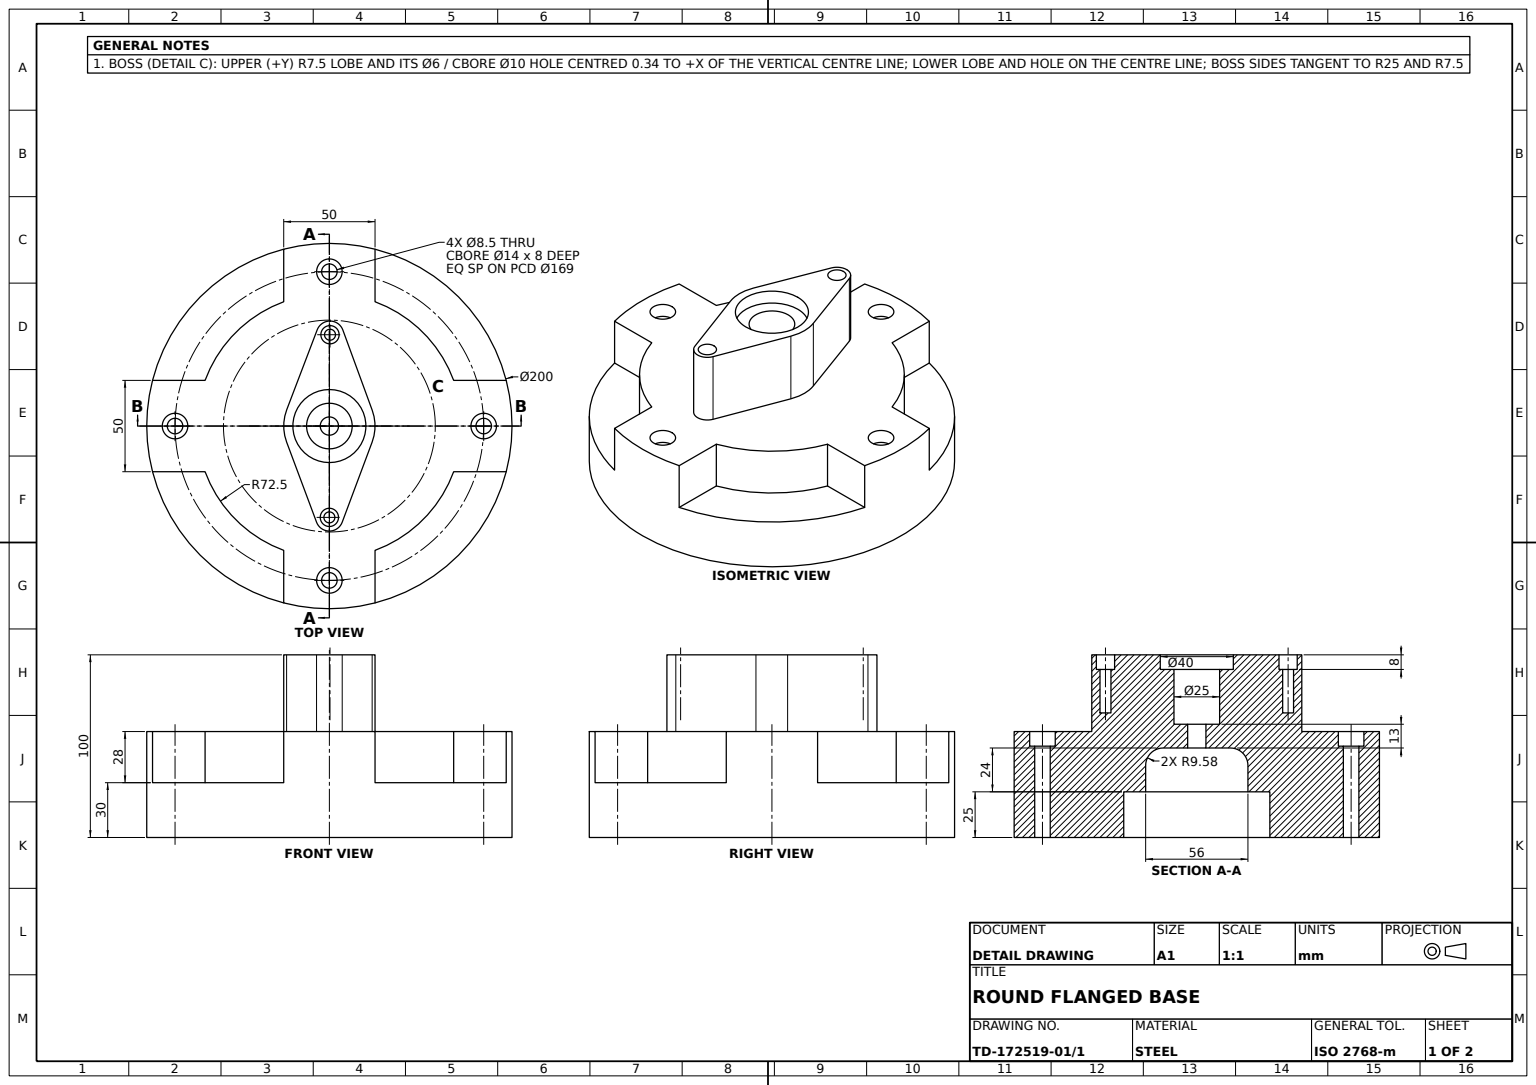
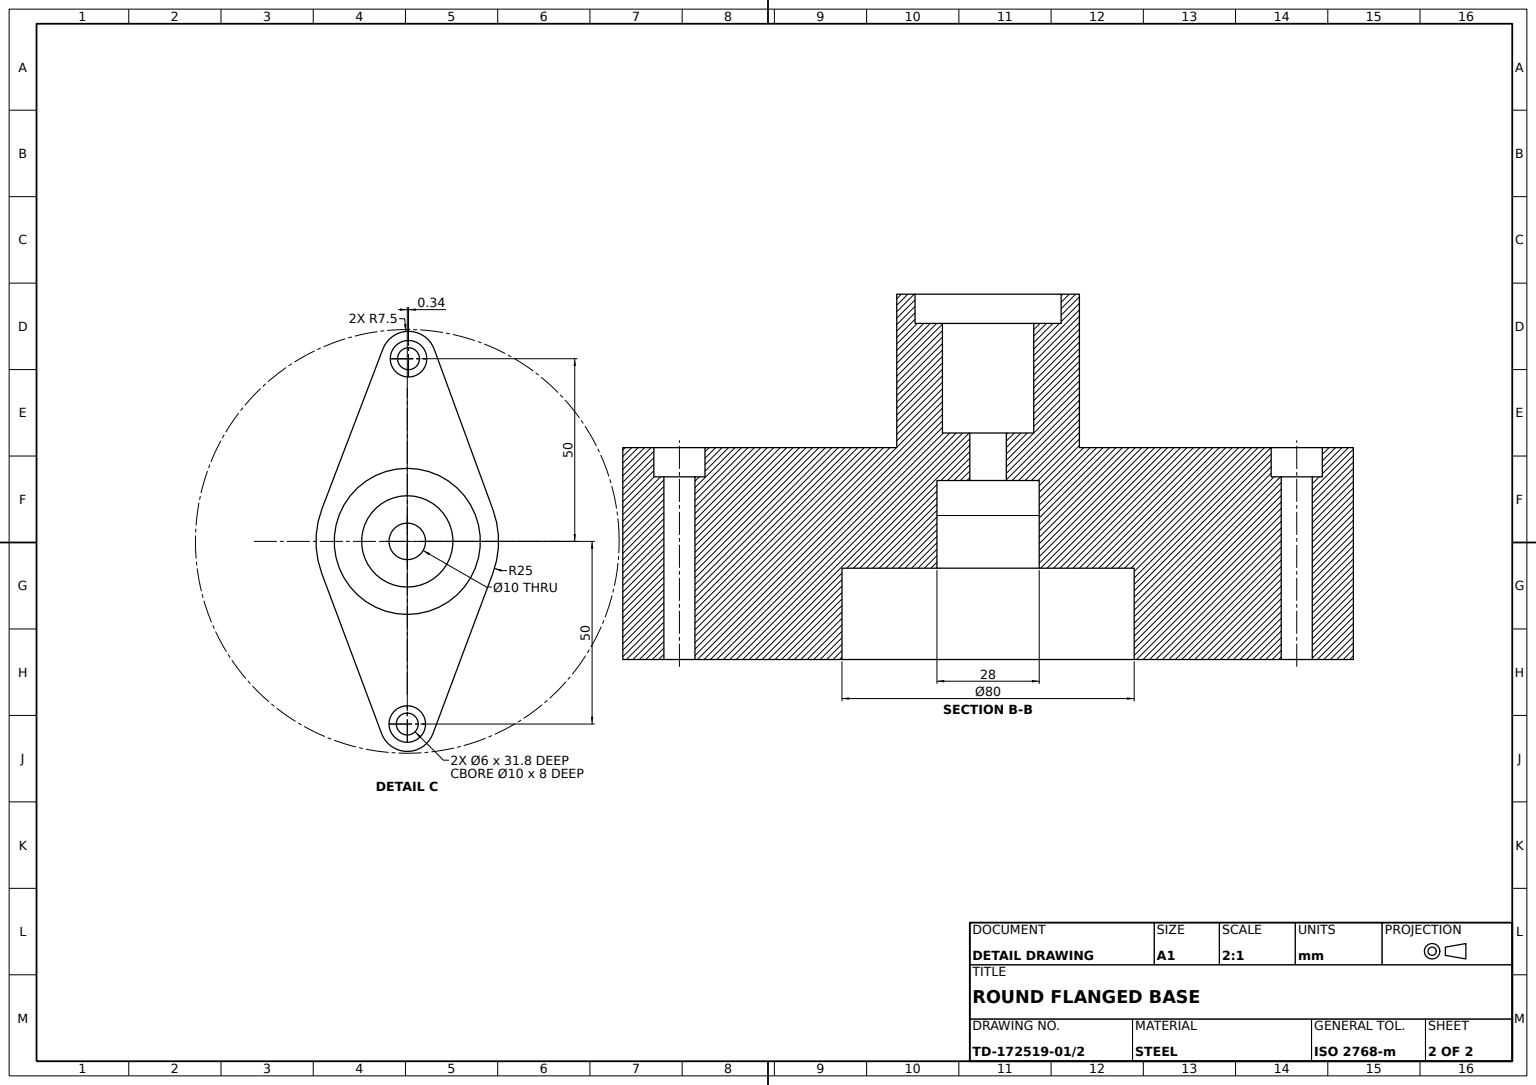
from build123d import *
from build123d.topology import SkipClean

# Parameters (mm, degrees)
BASE_FLANGE_SKETCH_R               = 100
BASE_FLANGE_200_DEPTH              = 30
MOUNTING_PAD_DEPTH                 = 28
MOUNTING_COUNTERBORES_SKETCH_R     = 7
MOUNTING_COUNTERBORES_4X_14_DEPTH  = 8
MOUNTING_HOLES_SKETCH_R            = 4.25
MOUNTING_HOLES_4X_8_5_DEPTH        = 50
SUPPORT_BOSS_DEPTH                 = 42
BEARING_COUNTERBORE_SKETCH_R       = 20
BEARING_COUNTERBORE_40_DEPTH       = 8
BEARING_BORE_SKETCH_R              = 12.5
BEARING_BORE_25_DEPTH              = 30
THROUGH_BORE_SKETCH_R              = 5
THROUGH_BORE_10_DEPTH              = 13
UNDERSIDE_RECESS_SKETCH_R          = 40
UNDERSIDE_RECESS_80_DEPTH          = 25
SIDE_SLOT_DEPTH                    = 14
BOSS_HOLE_COUNTERBORES_SKETCH_R    = 5
BOSS_HOLE_COUNTERBORES_2X_10_DEPTH = 8
BOSS_PIN_HOLES_SKETCH_R            = 3
BOSS_PIN_HOLES_2X_6_DEPTH          = 23.8


with BuildPart() as part:
    # Base Flange Sketch → Base Flange Ø200 (new body)
    with BuildSketch(Plane(origin=(0, 0, 0), x_dir=(1, 0, 0), z_dir=(0, 1, 0))):
        with Locations(Location((0, 0, 0), (0, 0, 270))):
            Circle(BASE_FLANGE_SKETCH_R)
    extrude(amount=BASE_FLANGE_200_DEPTH)

    # Mounting Pad Sketch → Mounting Pad (add)
    with SkipClean():  # the faces are left unmerged after this step: merging them gives an invalid solid
        with BuildSketch(Plane(origin=(0, 30, 0), x_dir=(1, 0, 0), z_dir=(0, 1, 0))):
            with BuildLine():
                Line((68.053287944, 25), (96.824583655, 25))
                ThreePointArc((96.824583655, 25), (100, 0), (96.824583655, -25))
                Line((96.824583655, -25), (68.053287944, -25))
                ThreePointArc((68.053287944, -25), (51.265241636, -51.265241636), (25, -68.053287944))
                Line((25, -68.053287944), (25, -96.824583655))
                ThreePointArc((25, -96.824583655), (0, -100), (-25, -96.824583655))
                Line((-25, -96.824583655), (-25, -68.053287944))
                ThreePointArc((-25, -68.053287944), (-51.265241636, -51.265241636), (-68.053287944, -25))
                Line((-68.053287944, -25), (-96.824583655, -25))
                ThreePointArc((-96.824583655, -25), (-100, 0), (-96.824583655, 25))
                Line((-96.824583655, 25), (-68.053287944, 25))
                ThreePointArc((-68.053287944, 25), (-51.265241636, 51.265241636), (-25, 68.053287944))
                Line((-25, 68.053287944), (-25, 96.824583655))
                ThreePointArc((-25, 96.824583655), (0, 100), (25, 96.824583655))
                Line((25, 96.824583655), (25, 68.053287944))
                ThreePointArc((25, 68.053287944), (51.265241636, 51.265241636), (68.053287944, 25))
            make_face()
        extrude(amount=MOUNTING_PAD_DEPTH)

    # Mounting Counterbores Sketch → Mounting Counterbores 4xØ14 (cut)
    with SkipClean():  # the faces are left unmerged after this step: merging them gives an invalid solid
        with BuildSketch(Plane(origin=(0, 58, 0), x_dir=(1, 0, 0), z_dir=(0, 1, 0))):
            with Locations(Location((0, 84.5, 0), (0, 0, 270))):
                Circle(MOUNTING_COUNTERBORES_SKETCH_R)
            with Locations(Location((84.5, 0, 0), (0, 0, 270))):
                Circle(MOUNTING_COUNTERBORES_SKETCH_R)
            with Locations(Location((0, -84.5, 0), (0, 0, 270))):
                Circle(MOUNTING_COUNTERBORES_SKETCH_R)
            with Locations(Location((-84.5, 0, 0), (0, 0, 270))):
                Circle(MOUNTING_COUNTERBORES_SKETCH_R)
        extrude(amount=-MOUNTING_COUNTERBORES_4X_14_DEPTH, mode=Mode.SUBTRACT)

    # Mounting Holes Sketch → Mounting Holes 4xØ8.5 (cut)
    with SkipClean():  # the faces are left unmerged after this step: merging them gives an invalid solid
        with BuildSketch(Plane(origin=(0, 50, 0), x_dir=(1, 0, 0), z_dir=(0, 1, 0))):
            with Locations(Location((0, 84.5, 0), (0, 0, 270))):
                Circle(MOUNTING_HOLES_SKETCH_R)
            with Locations(Location((84.5, 0, 0), (0, 0, 270))):
                Circle(MOUNTING_HOLES_SKETCH_R)
            with Locations(Location((0, -84.5, 0), (0, 0, 270))):
                Circle(MOUNTING_HOLES_SKETCH_R)
            with Locations(Location((-84.5, 0, 0), (0, 0, 270))):
                Circle(MOUNTING_HOLES_SKETCH_R)
        extrude(amount=-MOUNTING_HOLES_4X_8_5_DEPTH, mode=Mode.SUBTRACT)

    # Support Boss Sketch → Support Boss (add)
    with SkipClean():  # the faces are left unmerged after this step: merging them gives an invalid solid
        with BuildSketch(Plane(origin=(0, 58, 0), x_dir=(1, 0, 0), z_dir=(0, 1, 0))):
            with BuildLine():
                Line((-6.670404666, 52.671203723), (-23.359173661, 8.907805895))
                ThreePointArc((-23.359173661, 8.907805895), (-24.999857744, 0.084337338), (-23.418742494, -8.75))
                Line((-23.418742494, -8.75), (-7.025622749, -52.625))
                ThreePointArc((-7.025622749, -52.625), (-1e-09, -57.5), (7.025622747, -52.625))
                Line((7.025622747, -52.625), (23.418742494, -8.75))
                ThreePointArc((23.418742494, -8.75), (24.999857744, -0.084337338), (23.477245263, 8.591795789))
                Line((23.477245263, 8.591795789), (7.380521011, 52.576400691))
                ThreePointArc((7.380521011, 52.576400691), (0.387949547, 57.498691247), (-6.670404666, 52.671203723))
            make_face()
        extrude(amount=SUPPORT_BOSS_DEPTH)

    # Bearing Counterbore Sketch → Bearing Counterbore Ø40 (cut)
    with SkipClean():  # the faces are left unmerged after this step: merging them gives an invalid solid
        with BuildSketch(Plane(origin=(0, 100, 0), x_dir=(1, 0, 0), z_dir=(0, 1, 0))):
            with Locations(Location((0, 0, 0), (0, 0, 270))):
                Circle(BEARING_COUNTERBORE_SKETCH_R)
        extrude(amount=-BEARING_COUNTERBORE_40_DEPTH, mode=Mode.SUBTRACT)

    # Bearing Bore Sketch → Bearing Bore Ø25 (cut)
    with SkipClean():  # the faces are left unmerged after this step: merging them gives an invalid solid
        with BuildSketch(Plane(origin=(0, 92, 0), x_dir=(1, 0, 0), z_dir=(0, 1, 0))):
            with Locations(Location((0, 0, 0), (0, 0, 270))):
                Circle(BEARING_BORE_SKETCH_R)
        extrude(amount=-BEARING_BORE_25_DEPTH, mode=Mode.SUBTRACT)

    # Through Bore Sketch → Through Bore Ø10 (cut)
    with SkipClean():  # the faces are left unmerged after this step: merging them gives an invalid solid
        with BuildSketch(Plane(origin=(0, 62, 0), x_dir=(1, 0, 0), z_dir=(0, 1, 0))):
            with Locations(Location((0, 0, 0), (0, 0, 270))):
                Circle(THROUGH_BORE_SKETCH_R)
        extrude(amount=-THROUGH_BORE_10_DEPTH, mode=Mode.SUBTRACT)

    # Underside Recess Sketch → Underside Recess Ø80 (cut)
    with SkipClean():  # the faces are left unmerged after this step: merging them gives an invalid solid
        with BuildSketch(Plane.XZ):
            with Locations(Location((0, 0, 0), (0, 0, 270))):
                Circle(UNDERSIDE_RECESS_SKETCH_R)
        extrude(amount=-UNDERSIDE_RECESS_80_DEPTH, mode=Mode.SUBTRACT)

    # Side Slot Sketch → Side Slot (cut, symmetric)
    with SkipClean():  # the faces are left unmerged after this step: merging them gives an invalid solid
        with BuildSketch(Plane(origin=(0, 0, 0), x_dir=(0, 0, -1), z_dir=(1, 0, 0))):
            with BuildLine():
                Line((-28, 25), (28, 25))
                Line((28, 25), (28, 39.42))
                ThreePointArc((28, 39.42), (25.194082964, 46.194082964), (18.42, 49))
                Line((18.42, 49), (-18.42, 49))
                ThreePointArc((-18.42, 49), (-25.194082964, 46.194082964), (-28, 39.42))
                Line((-28, 39.42), (-28, 25))
            make_face()
        extrude(amount=SIDE_SLOT_DEPTH, both=True, mode=Mode.SUBTRACT)

    # Boss Hole Counterbores Sketch → Boss Hole Counterbores 2xØ10 (cut)
    with SkipClean():  # the faces are left unmerged after this step: merging them gives an invalid solid
        with BuildSketch(Plane(origin=(0, 100, 0), x_dir=(1, 0, 0), z_dir=(0, 1, 0))):
            with Locations(Location((0.337347432, 49.998861954, 0), (0, 0, 270))):
                Circle(BOSS_HOLE_COUNTERBORES_SKETCH_R)
            with Locations(Location((-1e-09, -50, 0), (0, 0, 270))):
                Circle(BOSS_HOLE_COUNTERBORES_SKETCH_R)
        extrude(amount=-BOSS_HOLE_COUNTERBORES_2X_10_DEPTH, mode=Mode.SUBTRACT)

    # Boss Pin Holes Sketch → Boss Pin Holes 2xØ6 (cut)
    with SkipClean():  # the faces are left unmerged after this step: merging them gives an invalid solid
        with BuildSketch(Plane(origin=(0, 92, 0), x_dir=(1, 0, 0), z_dir=(0, 1, 0))):
            with Locations(Location((0.337347432, 49.998861954, 0), (0, 0, 270))):
                Circle(BOSS_PIN_HOLES_SKETCH_R)
            with Locations(Location((-1e-09, -50, 0), (0, 0, 270))):
                Circle(BOSS_PIN_HOLES_SKETCH_R)
        extrude(amount=-BOSS_PIN_HOLES_2X_6_DEPTH, mode=Mode.SUBTRACT)


solid = part.part
